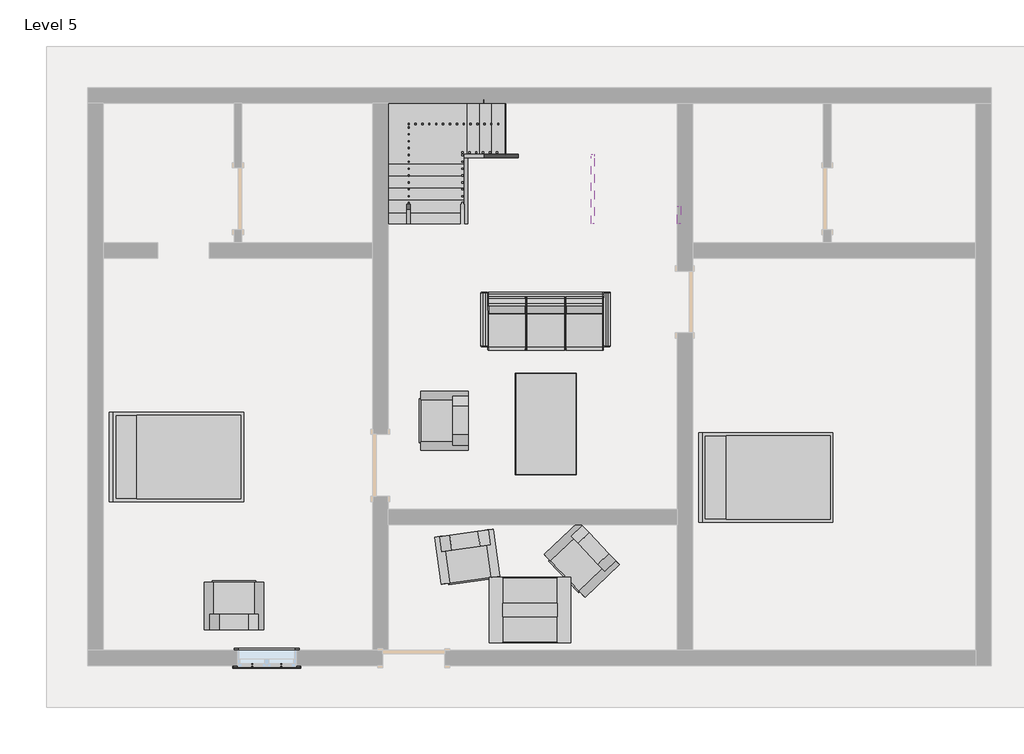
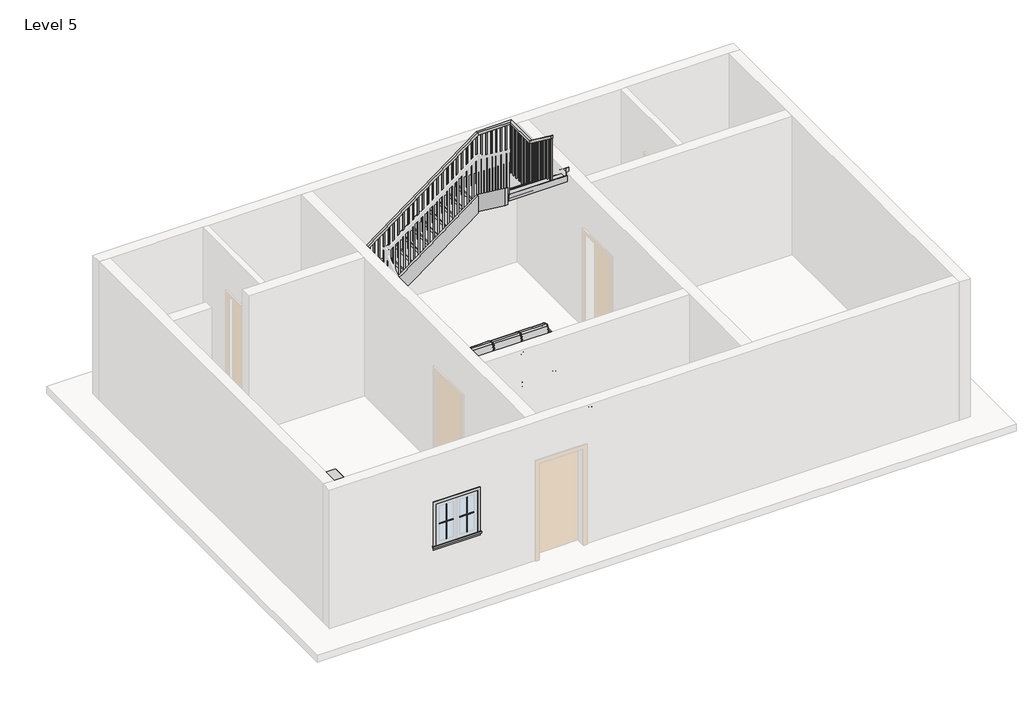
# One storey, part 2 of 2: 9 furniture elements, 6 members, 4 proxies, 1 railing, 1 stair flight.
"""IFC4 building model written with IfcOpenShell, lengths in millimetres."""

from ifc_helpers import new_model, si_unit, frame, origin, place, context, project, spatial, polyline, outline, extrude, faceted_brep, transform, mapped, element, save
from components import muntin_pattern_2x2_muntin_pattern_2x2_b3fe6957, muntin_pattern_2x2_muntin_pattern_2x2_3e0ecaf2, trim_window_exterior_flat_with_sill_41619996, trim_window_interior_flat_picture_frame_51c85655, furniture_2fc85b74, furniture_29a9adb8, furniture_57072a26, bed_17739_bed_17739_15c61121, chair_lounge_11461_couch_0866092f, dining_table_14755_dining_table_14755_d89cb775, wood_and_glass_coffee_table_17065_wood_and_glass_coffee_dbc724b2, stair_flight_e836c5a9

model = new_model("IFC4")

# Units and contexts
model_context = context("Model", 3, world=origin())
ifc_project = project(units=[si_unit("LENGTHUNIT", "METRE", prefix="MILLI")], contexts=[model_context])

# Site, building, storey
site = spatial("IfcSite", under=ifc_project)
building = spatial("IfcBuilding", under=site)
storey = spatial("IfcBuildingStorey", under=building, Name="Level 5", Elevation=9601.2)

# Proxies
placement = place(None, origin())
muntin_pattern_2x2_muntin_pattern_2x2_shape = muntin_pattern_2x2_muntin_pattern_2x2_b3fe6957(model_context)
element("IfcBuildingElementProxy", 1, Name="Muntin Pattern_2x2 : Muntin Pattern_2x2", ObjectType="Muntin Pattern_2x2 : Muntin Pattern_2x2", at=placement, inside=storey, context=model_context, shape_type="MappedRepresentation", body=[
    mapped(muntin_pattern_2x2_muntin_pattern_2x2_shape, transform((-5069.3921642, -1799.3582394, 10738.1934313), x_axis=(-1.0, 0.0, 0.0), y_axis=(0.0, -1.0, 0.0), z_axis=(0.0, 0.0, 1.0))),
])
muntin_pattern_2x2_muntin_pattern_2x2_2_shape = muntin_pattern_2x2_muntin_pattern_2x2_3e0ecaf2(model_context)
element("IfcBuildingElementProxy", 2, Name="Muntin Pattern_2x2 : Muntin Pattern_2x2", ObjectType="Muntin Pattern_2x2 : Muntin Pattern_2x2", at=placement, inside=storey, context=model_context, shape_type="MappedRepresentation", body=[
    mapped(muntin_pattern_2x2_muntin_pattern_2x2_2_shape, transform((-5498.0171642, -1799.3582394, 10738.1934313), x_axis=(1.0, 0.0, 0.0), y_axis=(0.0, 1.0, 0.0), z_axis=(0.0, 0.0, 1.0))),
])
trim_window_exterior_flat_with_sill_shape = trim_window_exterior_flat_with_sill_41619996(model_context)
element("IfcBuildingElementProxy", 3, Name="Trim-Window-Exterior-Flat : with Sill", ObjectType="Trim-Window-Exterior-Flat : with Sill", at=placement, inside=storey, context=model_context, shape_type="MappedRepresentation", body=[
    mapped(trim_window_exterior_flat_with_sill_shape, transform((-5283.7046642, -1808.8832394, 11582.7434313), x_axis=(1.0, 0.0, 0.0), y_axis=(0.0, 0.0, 1.0), z_axis=(0.0, -1.0, 0.0))),
])
trim_window_interior_flat_picture_frame_shape = trim_window_interior_flat_picture_frame_51c85655(model_context)
element("IfcBuildingElementProxy", 4, Name="Trim-Window-Interior-Flat : Picture Frame", ObjectType="Trim-Window-Interior-Flat : Picture Frame", at=placement, inside=storey, context=model_context, shape_type="MappedRepresentation", body=[
    mapped(trim_window_interior_flat_picture_frame_shape, transform((-5283.7046642, -1580.2832394, 11582.7434313), x_axis=(-1.0, 0.0, 0.0), y_axis=(0.0, 0.0, 1.0), z_axis=(0.0, 1.0, 0.0))),
])

# Furniture
furniture_shape = furniture_2fc85b74(model_context)
furniture_2_shape = furniture_29a9adb8(model_context)
furniture_3_shape = furniture_57072a26(model_context)
element("IfcFurniture", 5, at=placement, inside=storey, context=model_context, shape_type="MappedRepresentation", body=[
    mapped(furniture_shape, transform((-1166.392994, 2905.4688314, 9601.2), x_axis=(1.0, 0.0, 0.0), y_axis=(0.0, 1.0, 0.0), z_axis=(0.0, 0.0, 1.0))),
    mapped(furniture_2_shape, transform((-1166.392994, 2905.4688314, 9601.2), x_axis=(1.0, 0.0, 0.0), y_axis=(0.0, 1.0, 0.0), z_axis=(0.0, 0.0, 1.0))),
    mapped(furniture_3_shape, transform((-1166.392994, 2905.4688314, 9601.2), x_axis=(1.0, 0.0, 0.0), y_axis=(0.0, 1.0, 0.0), z_axis=(0.0, 0.0, 1.0))),
])
bed_17739_bed_17739_shape = bed_17739_bed_17739_15c61121(model_context)
element("IfcFurniture", 6, ObjectType="Bed_17739 : Bed_17739", at=placement, inside=storey, context=model_context, shape_type="MappedRepresentation", body=[
    mapped(bed_17739_bed_17739_shape, transform((-6591.8046642, 1277.2167606, 9601.2), x_axis=(0.0, 1.0, 0.0), y_axis=(-1.0, 0.0, 0.0), z_axis=(0.0, 0.0, 1.0))),
])
element("IfcFurniture", 7, ObjectType="Bed_17739 : Bed_17739", at=placement, inside=storey, context=model_context, shape_type="MappedRepresentation", body=[
    mapped(bed_17739_bed_17739_shape, transform((2107.6953358, 972.4167606, 9601.2), x_axis=(0.0, 1.0, 0.0), y_axis=(-1.0, 0.0, 0.0), z_axis=(0.0, 0.0, 1.0))),
])
chair_lounge_11461_couch_shape = chair_lounge_11461_couch_0866092f(model_context)
element("IfcFurniture", 8, ObjectType="Chair-Lounge_11461 : Couch", at=placement, inside=storey, context=model_context, shape_type="MappedRepresentation", body=[
    mapped(chair_lounge_11461_couch_shape, transform((-5766.3046642, -1273.9095448, 9601.2), x_axis=(-1.0, 0.0, 0.0), y_axis=(0.0, -1.0, 0.0), z_axis=(0.0, 0.0, 1.0))),
])
element("IfcFurniture", 9, ObjectType="Chair-Lounge_11461 : Couch", at=placement, inside=storey, context=model_context, shape_type="MappedRepresentation", body=[
    mapped(chair_lounge_11461_couch_shape, transform((-2311.9046642, 1810.6167606, 9601.2), x_axis=(0.0, -1.0, 0.0), y_axis=(1.0, 0.0, 0.0), z_axis=(0.0, 0.0, 1.0))),
])
element("IfcFurniture", 10, ObjectType="Chair-Lounge_11461 : Couch", at=placement, inside=storey, context=model_context, shape_type="MappedRepresentation", body=[
    mapped(chair_lounge_11461_couch_shape, transform((-2372.9488995, 149.9169276, 9601.2), x_axis=(0.9905324493396854, 0.1372787922627668, 0.0), y_axis=(-0.1372787922627668, 0.9905324493396854, 0.0), z_axis=(0.0, 0.0, 1.0))),
])
element("IfcFurniture", 11, ObjectType="Chair-Lounge_11461 : Couch", at=placement, inside=storey, context=model_context, shape_type="MappedRepresentation", body=[
    mapped(chair_lounge_11461_couch_shape, transform((-378.7925234, 1.7617886, 9601.2), x_axis=(0.6894995564131732, -0.7242861048688133, 0.0), y_axis=(0.7242861048688133, 0.6894995564131732, 0.0), z_axis=(0.0, 0.0, 1.0))),
])
dining_table_14755_dining_table_14755_shape = dining_table_14755_dining_table_14755_d89cb775(model_context)
element("IfcFurniture", 12, ObjectType="Dining_table_14755 : Dining_table_14755", at=placement, inside=storey, context=model_context, shape_type="MappedRepresentation", body=[
    mapped(dining_table_14755_dining_table_14755_shape, transform((-711.7046642, 1010.5167606, 9601.2), x_axis=(0.0, 1.0, 0.0), y_axis=(-1.0, 0.0, 0.0), z_axis=(0.0, 0.0, 1.0))),
])
wood_and_glass_coffee_table_17065_wood_and_glass_coffee_shape = wood_and_glass_coffee_table_17065_wood_and_glass_coffee_dbc724b2(model_context)
element("IfcFurniture", 13, ObjectType="Wood_and_Glass_Coffee_Table_17065 : Wood_and_Glass_Coffee_Table_17065", at=placement, inside=storey, context=model_context, shape_type="MappedRepresentation", body=[
    mapped(wood_and_glass_coffee_table_17065_wood_and_glass_coffee_shape, transform((-1397.5046642, -983.3832394, 9601.2), x_axis=(1.0, 0.0, 0.0), y_axis=(0.0, 1.0, 0.0), z_axis=(0.0, 0.0, 1.0))),
])

# Members
element("IfcMember", 14, ObjectType="Stringer - 2\" Width", at=placement, inside=storey, context=model_context, shape_type="SweptSolid", body=[
    extrude(outline(polyline([(4718.9167606, 9601.2), (4718.9167606, 9748.8508226), (5113.281957, 9748.8508226), (4911.6463024, 9601.2), (4718.9167606, 9601.2)])), frame((-3543.8046642, 0.0, 0.0), z_axis=(1.0, 0.0, 0.0), x_axis=(0.0, 1.0, 0.0)), (0.0, 0.0, 1.0), 50.8),
])
element("IfcMember", 15, ObjectType="Stringer - 2\" Width", at=placement, inside=storey, context=model_context, shape_type="SweptSolid", body=[
    extrude(outline(polyline([(10762.0387795, -1623.6098785), (11417.9484291, -743.5977653), (11417.9484291, -1253.6320422), (10762.0387795, -2133.6441554), (10762.0387795, -1623.6098785)])), frame((0.0, 6496.9167606, 0.0), z_axis=(0.0, 1.0, 0.0), x_axis=(0.0, 0.0, 1.0)), (0.0, 0.0, 1.0), 50.8),
])
element("IfcMember", 16, ObjectType="Stringer - 2\" Width", at=placement, inside=storey, context=model_context, shape_type="SweptSolid", body=[
    extrude(outline(polyline([(4718.9167606, 12549.2227901), (4718.9167606, 12743.1652405), (4979.1229954, 12549.2227901), (4718.9167606, 12549.2227901)])), frame((774.1953358, 0.0, 0.0), z_axis=(1.0, 0.0, 0.0), x_axis=(0.0, 1.0, 0.0)), (0.0, 0.0, 1.0), 50.8),
])
element("IfcMember", 17, ObjectType="Stringer - 2\" Width", at=placement, inside=storey, context=model_context, shape_type="SweptSolid", body=[
    extrude(outline(polyline([(4718.9167606, 9601.2), (4718.9167606, 9837.8522719), (5695.7536537, 10553.1561753), (5695.7536537, 10175.3747195), (4911.6463024, 9601.2), (4718.9167606, 9601.2)])), frame((-2368.6972892, 0.0, 0.0), z_axis=(1.0, 0.0, 0.0), x_axis=(0.0, 1.0, 0.0)), (0.0, 0.0, 1.0), 50.8),
])
element("IfcMember", 18, ObjectType="Stringer - 2\" Width", at=placement, inside=storey, context=model_context, shape_type="SweptSolid", body=[
    extrude(outline(polyline([(10586.8438971, -2368.6972892), (10212.5738041, -2368.6972892), (10212.5738041, -2360.8087204), (11602.6389392, -495.8046642), (11977.2250342, -495.8046642), (11977.2250342, -503.2692636), (10586.8438971, -2368.6972892)])), frame((0.0, 5695.7536537, 0.0), z_axis=(0.0, 1.0, 0.0), x_axis=(0.0, 0.0, 1.0)), (0.0, 0.0, 1.0), 50.8),
])
element("IfcMember", 19, ObjectType="Stringer - 2\" Width", at=placement, inside=storey, context=model_context, shape_type="SweptSolid", body=[
    extrude(outline(polyline([(5746.5536537, 11977.2250342), (5746.5536537, 11640.5022932), (5688.2891085, 11640.5022932), (4718.9167606, 12363.0155283), (4718.9167606, 12743.1652405), (5746.5536537, 11977.2250342)])), frame((-495.8046642, 0.0, 0.0), z_axis=(1.0, 0.0, 0.0), x_axis=(0.0, 1.0, 0.0)), (0.0, 0.0, 1.0), 50.8),
])

# Railing
element("IfcRailing", 20, ObjectType="Handrail - Rectangular", at=placement, inside=storey, context=model_context, shape_type="SolidModel", body=[
    faceted_brep([(-3213.6046642, 4718.9167606, 10648.1217391), (-3213.6046642, 4718.9167606, 10584.7634439), (-3162.8046642, 4718.9167606, 10584.7634439), (-3162.8046642, 4718.9167606, 10648.1217391), (-3213.6046642, 5555.0306195, 11271.312193), (-3213.6046642, 5571.8796657, 11220.512193), (-3162.8046642, 5571.8796657, 11220.512193), (-3162.8046642, 5555.0306195, 11271.312193), (-3213.6046642, 6217.5167606, 11271.312193), (-3213.6046642, 6217.5167606, 11220.512193), (-3162.8046642, 6166.7167606, 11220.512193), (-3162.8046642, 6166.7167606, 11271.312193), (-2551.1185231, 6217.5167606, 11271.312193), (-2534.269477, 6217.5167606, 11220.512193), (-2534.269477, 6166.7167606, 11220.512193), (-2551.1185231, 6166.7167606, 11271.312193), (-239.7185231, 6217.5167606, 12994.0948017), (-222.869477, 6217.5167606, 12943.2948017), (-222.869477, 6166.7167606, 12943.2948017), (-239.7185231, 6166.7167606, 12994.0948017), (494.7953358, 6217.5167606, 12994.0948017), (494.7953358, 6217.5167606, 12943.2948017), (443.9953358, 6166.7167606, 12943.2948017), (443.9953358, 6166.7167606, 12994.0948017), (494.7953358, 5483.0029017, 12994.0948017), (494.7953358, 5466.1538556, 12943.2948017), (443.9953358, 5466.1538556, 12943.2948017), (443.9953358, 5483.0029017, 12994.0948017), (494.7953358, 4718.9167606, 13563.6), (443.9953358, 4718.9167606, 13563.6), (443.9953358, 4718.9167606, 13500.2417047), (494.7953358, 4718.9167606, 13500.2417047)], [[[0, 1, 2, 3]], [[1, 0, 4, 5]], [[2, 1, 5, 6]], [[3, 2, 6, 7]], [[0, 3, 7, 4]], [[5, 4, 8, 9]], [[6, 5, 9, 10]], [[7, 6, 10, 11]], [[4, 7, 11, 8]], [[9, 8, 12, 13]], [[10, 9, 13, 14]], [[11, 10, 14, 15]], [[8, 11, 15, 12]], [[13, 12, 16, 17]], [[14, 13, 17, 18]], [[15, 14, 18, 19]], [[12, 15, 19, 16]], [[17, 16, 20, 21]], [[18, 17, 21, 22]], [[19, 18, 22, 23]], [[16, 19, 23, 20]], [[21, 20, 24, 25]], [[22, 21, 25, 26]], [[23, 22, 26, 27]], [[20, 23, 27, 24]], [[28, 29, 30, 31]], [[25, 24, 28, 31]], [[26, 25, 31, 30]], [[27, 26, 30, 29]], [[24, 27, 29, 28]]]),
    extrude(outline(polyline([(4779.2417606, 13455.2789718), (4779.2417606, 12516.6782609), (4760.1917606, 12516.6782609), (4760.1917606, 13469.4777296), (4779.2417606, 13455.2789718)])), frame((459.8703358, 0.0, 0.0), z_axis=(1.0, 0.0, 0.0), x_axis=(0.0, 1.0, 0.0)), (0.0, 0.0, 1.0), 19.05),
    extrude(outline(polyline([(4880.8417606, 13379.5522637), (4880.8417606, 12516.6782609), (4861.7917606, 12516.6782609), (4861.7917606, 13393.7510215), (4880.8417606, 13379.5522637)])), frame((459.8703358, 0.0, 0.0), z_axis=(1.0, 0.0, 0.0), x_axis=(0.0, 1.0, 0.0)), (0.0, 0.0, 1.0), 19.05),
    extrude(outline(polyline([(4982.4417606, 13303.8255557), (4982.4417606, 12384.1565217), (4963.3917606, 12384.1565217), (4963.3917606, 13318.0243134), (4982.4417606, 13303.8255557)])), frame((459.8703358, 0.0, 0.0), z_axis=(1.0, 0.0, 0.0), x_axis=(0.0, 1.0, 0.0)), (0.0, 0.0, 1.0), 19.05),
    extrude(outline(polyline([(5084.0417606, 13228.0988476), (5084.0417606, 12384.1565217), (5064.9917606, 12384.1565217), (5064.9917606, 13242.2976054), (5084.0417606, 13228.0988476)])), frame((459.8703358, 0.0, 0.0), z_axis=(1.0, 0.0, 0.0), x_axis=(0.0, 1.0, 0.0)), (0.0, 0.0, 1.0), 19.05),
    extrude(outline(polyline([(5185.6417606, 13152.3721395), (5185.6417606, 12251.6347826), (5166.5917606, 12251.6347826), (5166.5917606, 13166.5708973), (5185.6417606, 13152.3721395)])), frame((459.8703358, 0.0, 0.0), z_axis=(1.0, 0.0, 0.0), x_axis=(0.0, 1.0, 0.0)), (0.0, 0.0, 1.0), 19.05),
    extrude(outline(polyline([(5287.2417606, 13076.6454314), (5287.2417606, 12119.1130435), (5268.1917606, 12119.1130435), (5268.1917606, 13090.8441892), (5287.2417606, 13076.6454314)])), frame((459.8703358, 0.0, 0.0), z_axis=(1.0, 0.0, 0.0), x_axis=(0.0, 1.0, 0.0)), (0.0, 0.0, 1.0), 19.05),
    extrude(outline(polyline([(5388.8417606, 13000.9187234), (5388.8417606, 12119.1130435), (5369.7917606, 12119.1130435), (5369.7917606, 13015.1174811), (5388.8417606, 13000.9187234)])), frame((459.8703358, 0.0, 0.0), z_axis=(1.0, 0.0, 0.0), x_axis=(0.0, 1.0, 0.0)), (0.0, 0.0, 1.0), 19.05),
    extrude(outline(polyline([(5490.4417606, 12925.1920153), (5490.4417606, 11986.5913043), (5471.3917606, 11986.5913043), (5471.3917606, 12939.3907731), (5490.4417606, 12925.1920153)])), frame((459.8703358, 0.0, 0.0), z_axis=(1.0, 0.0, 0.0), x_axis=(0.0, 1.0, 0.0)), (0.0, 0.0, 1.0), 19.05),
    extrude(outline(polyline([(478.9203358, 5592.0417606), (478.9203358, 5572.9917606), (459.8703358, 5572.9917606), (459.8703358, 5592.0417606), (478.9203358, 5592.0417606)])), frame((0.0, 0.0, 11986.5913043), z_axis=(0.0, 0.0, 1.0), x_axis=(1.0, 0.0, 0.0)), (0.0, 0.0, 1.0), 956.7034973),
    extrude(outline(polyline([(478.9203358, 5693.6417606), (478.9203358, 5674.5917606), (459.8703358, 5674.5917606), (459.8703358, 5693.6417606), (478.9203358, 5693.6417606)])), frame((0.0, 0.0, 11854.0695652), z_axis=(0.0, 0.0, 1.0), x_axis=(1.0, 0.0, 0.0)), (0.0, 0.0, 1.0), 1089.2252364),
    extrude(outline(polyline([(478.9203358, 5795.2417606), (478.9203358, 5776.1917606), (459.8703358, 5776.1917606), (459.8703358, 5795.2417606), (478.9203358, 5795.2417606)])), frame((0.0, 0.0, 11854.0695652), z_axis=(0.0, 0.0, 1.0), x_axis=(1.0, 0.0, 0.0)), (0.0, 0.0, 1.0), 1089.2252364),
    extrude(outline(polyline([(478.9203358, 5896.8417606), (478.9203358, 5877.7917606), (459.8703358, 5877.7917606), (459.8703358, 5896.8417606), (478.9203358, 5896.8417606)])), frame((0.0, 0.0, 11854.0695652), z_axis=(0.0, 0.0, 1.0), x_axis=(1.0, 0.0, 0.0)), (0.0, 0.0, 1.0), 1089.2252364),
    extrude(outline(polyline([(478.9203358, 5998.4417606), (478.9203358, 5979.3917606), (459.8703358, 5979.3917606), (459.8703358, 5998.4417606), (478.9203358, 5998.4417606)])), frame((0.0, 0.0, 11854.0695652), z_axis=(0.0, 0.0, 1.0), x_axis=(1.0, 0.0, 0.0)), (0.0, 0.0, 1.0), 1089.2252364),
    extrude(outline(polyline([(478.9203358, 6100.0417606), (478.9203358, 6080.9917606), (459.8703358, 6080.9917606), (459.8703358, 6100.0417606), (478.9203358, 6100.0417606)])), frame((0.0, 0.0, 11854.0695652), z_axis=(0.0, 0.0, 1.0), x_axis=(1.0, 0.0, 0.0)), (0.0, 0.0, 1.0), 1089.2252364),
    extrude(outline(polyline([(358.2703358, 6201.6417606), (377.3203358, 6201.6417606), (377.3203358, 6182.5917606), (358.2703358, 6182.5917606), (358.2703358, 6201.6417606)])), frame((0.0, 0.0, 11854.0695652), z_axis=(0.0, 0.0, 1.0), x_axis=(1.0, 0.0, 0.0)), (0.0, 0.0, 1.0), 1089.2252364),
    extrude(outline(polyline([(256.6703358, 6201.6417606), (275.7203358, 6201.6417606), (275.7203358, 6182.5917606), (256.6703358, 6182.5917606), (256.6703358, 6201.6417606)])), frame((0.0, 0.0, 11854.0695652), z_axis=(0.0, 0.0, 1.0), x_axis=(1.0, 0.0, 0.0)), (0.0, 0.0, 1.0), 1089.2252364),
    extrude(outline(polyline([(155.0703358, 6201.6417606), (174.1203358, 6201.6417606), (174.1203358, 6182.5917606), (155.0703358, 6182.5917606), (155.0703358, 6201.6417606)])), frame((0.0, 0.0, 11854.0695652), z_axis=(0.0, 0.0, 1.0), x_axis=(1.0, 0.0, 0.0)), (0.0, 0.0, 1.0), 1089.2252364),
    extrude(outline(polyline([(53.4703358, 6201.6417606), (72.5203358, 6201.6417606), (72.5203358, 6182.5917606), (53.4703358, 6182.5917606), (53.4703358, 6201.6417606)])), frame((0.0, 0.0, 11854.0695652), z_axis=(0.0, 0.0, 1.0), x_axis=(1.0, 0.0, 0.0)), (0.0, 0.0, 1.0), 1089.2252364),
    extrude(outline(polyline([(-48.1296642, 6201.6417606), (-29.0796642, 6201.6417606), (-29.0796642, 6182.5917606), (-48.1296642, 6182.5917606), (-48.1296642, 6201.6417606)])), frame((0.0, 0.0, 11854.0695652), z_axis=(0.0, 0.0, 1.0), x_axis=(1.0, 0.0, 0.0)), (0.0, 0.0, 1.0), 1089.2252364),
    extrude(outline(polyline([(-149.7296642, 6201.6417606), (-130.6796642, 6201.6417606), (-130.6796642, 6182.5917606), (-149.7296642, 6182.5917606), (-149.7296642, 6201.6417606)])), frame((0.0, 0.0, 11854.0695652), z_axis=(0.0, 0.0, 1.0), x_axis=(1.0, 0.0, 0.0)), (0.0, 0.0, 1.0), 1089.2252364),
    extrude(outline(polyline([(12922.0822397, -251.3296642), (11854.0695652, -251.3296642), (11854.0695652, -232.2796642), (12936.2809975, -232.2796642), (12922.0822397, -251.3296642)])), frame((0.0, 6182.5917606, 0.0), z_axis=(0.0, 1.0, 0.0), x_axis=(0.0, 0.0, 1.0)), (0.0, 0.0, 1.0), 19.05),
    extrude(outline(polyline([(12846.3555316, -352.9296642), (11854.0695652, -352.9296642), (11854.0695652, -333.8796642), (12860.5542894, -333.8796642), (12846.3555316, -352.9296642)])), frame((0.0, 6182.5917606, 0.0), z_axis=(0.0, 1.0, 0.0), x_axis=(0.0, 0.0, 1.0)), (0.0, 0.0, 1.0), 19.05),
    extrude(outline(polyline([(12770.6288236, -454.5296642), (11854.0695652, -454.5296642), (11854.0695652, -435.4796642), (12784.8275813, -435.4796642), (12770.6288236, -454.5296642)])), frame((0.0, 6182.5917606, 0.0), z_axis=(0.0, 1.0, 0.0), x_axis=(0.0, 0.0, 1.0)), (0.0, 0.0, 1.0), 19.05),
    extrude(outline(polyline([(12694.9021155, -556.1296642), (11721.5478261, -556.1296642), (11721.5478261, -537.0796642), (12709.1008733, -537.0796642), (12694.9021155, -556.1296642)])), frame((0.0, 6182.5917606, 0.0), z_axis=(0.0, 1.0, 0.0), x_axis=(0.0, 0.0, 1.0)), (0.0, 0.0, 1.0), 19.05),
    extrude(outline(polyline([(12619.1754074, -657.7296642), (11721.5478261, -657.7296642), (11721.5478261, -638.6796642), (12633.3741652, -638.6796642), (12619.1754074, -657.7296642)])), frame((0.0, 6182.5917606, 0.0), z_axis=(0.0, 1.0, 0.0), x_axis=(0.0, 0.0, 1.0)), (0.0, 0.0, 1.0), 19.05),
    extrude(outline(polyline([(12543.4486993, -759.3296642), (11589.026087, -759.3296642), (11589.026087, -740.2796642), (12557.6474571, -740.2796642), (12543.4486993, -759.3296642)])), frame((0.0, 6182.5917606, 0.0), z_axis=(0.0, 1.0, 0.0), x_axis=(0.0, 0.0, 1.0)), (0.0, 0.0, 1.0), 19.05),
    extrude(outline(polyline([(12467.7219913, -860.9296642), (11589.026087, -860.9296642), (11589.026087, -841.8796642), (12481.920749, -841.8796642), (12467.7219913, -860.9296642)])), frame((0.0, 6182.5917606, 0.0), z_axis=(0.0, 1.0, 0.0), x_axis=(0.0, 0.0, 1.0)), (0.0, 0.0, 1.0), 19.05),
    extrude(outline(polyline([(12391.9952832, -962.5296642), (11456.5043478, -962.5296642), (11456.5043478, -943.4796642), (12406.194041, -943.4796642), (12391.9952832, -962.5296642)])), frame((0.0, 6182.5917606, 0.0), z_axis=(0.0, 1.0, 0.0), x_axis=(0.0, 0.0, 1.0)), (0.0, 0.0, 1.0), 19.05),
    extrude(outline(polyline([(12316.2685751, -1064.1296642), (11456.5043478, -1064.1296642), (11456.5043478, -1045.0796642), (12330.4673329, -1045.0796642), (12316.2685751, -1064.1296642)])), frame((0.0, 6182.5917606, 0.0), z_axis=(0.0, 1.0, 0.0), x_axis=(0.0, 0.0, 1.0)), (0.0, 0.0, 1.0), 19.05),
    extrude(outline(polyline([(12240.541867, -1165.7296642), (11323.9826087, -1165.7296642), (11323.9826087, -1146.6796642), (12254.7406248, -1146.6796642), (12240.541867, -1165.7296642)])), frame((0.0, 6182.5917606, 0.0), z_axis=(0.0, 1.0, 0.0), x_axis=(0.0, 0.0, 1.0)), (0.0, 0.0, 1.0), 19.05),
    extrude(outline(polyline([(12164.815159, -1267.3296642), (11191.4608696, -1267.3296642), (11191.4608696, -1248.2796642), (12179.0139167, -1248.2796642), (12164.815159, -1267.3296642)])), frame((0.0, 6182.5917606, 0.0), z_axis=(0.0, 1.0, 0.0), x_axis=(0.0, 0.0, 1.0)), (0.0, 0.0, 1.0), 19.05),
    extrude(outline(polyline([(12089.0884509, -1368.9296642), (11191.4608696, -1368.9296642), (11191.4608696, -1349.8796642), (12103.2872087, -1349.8796642), (12089.0884509, -1368.9296642)])), frame((0.0, 6182.5917606, 0.0), z_axis=(0.0, 1.0, 0.0), x_axis=(0.0, 0.0, 1.0)), (0.0, 0.0, 1.0), 19.05),
    extrude(outline(polyline([(12013.3617428, -1470.5296642), (11058.9391304, -1470.5296642), (11058.9391304, -1451.4796642), (12027.5605006, -1451.4796642), (12013.3617428, -1470.5296642)])), frame((0.0, 6182.5917606, 0.0), z_axis=(0.0, 1.0, 0.0), x_axis=(0.0, 0.0, 1.0)), (0.0, 0.0, 1.0), 19.05),
    extrude(outline(polyline([(11937.6350347, -1572.1296642), (11058.9391304, -1572.1296642), (11058.9391304, -1553.0796642), (11951.8337925, -1553.0796642), (11937.6350347, -1572.1296642)])), frame((0.0, 6182.5917606, 0.0), z_axis=(0.0, 1.0, 0.0), x_axis=(0.0, 0.0, 1.0)), (0.0, 0.0, 1.0), 19.05),
    extrude(outline(polyline([(11861.9083267, -1673.7296642), (10926.4173913, -1673.7296642), (10926.4173913, -1654.6796642), (11876.1070844, -1654.6796642), (11861.9083267, -1673.7296642)])), frame((0.0, 6182.5917606, 0.0), z_axis=(0.0, 1.0, 0.0), x_axis=(0.0, 0.0, 1.0)), (0.0, 0.0, 1.0), 19.05),
    extrude(outline(polyline([(11786.1816186, -1775.3296642), (10926.4173913, -1775.3296642), (10926.4173913, -1756.2796642), (11800.3803764, -1756.2796642), (11786.1816186, -1775.3296642)])), frame((0.0, 6182.5917606, 0.0), z_axis=(0.0, 1.0, 0.0), x_axis=(0.0, 0.0, 1.0)), (0.0, 0.0, 1.0), 19.05),
    extrude(outline(polyline([(11710.4549105, -1876.9296642), (10793.8956522, -1876.9296642), (10793.8956522, -1857.8796642), (11724.6536683, -1857.8796642), (11710.4549105, -1876.9296642)])), frame((0.0, 6182.5917606, 0.0), z_axis=(0.0, 1.0, 0.0), x_axis=(0.0, 0.0, 1.0)), (0.0, 0.0, 1.0), 19.05),
    extrude(outline(polyline([(11634.7282025, -1978.5296642), (10661.373913, -1978.5296642), (10661.373913, -1959.4796642), (11648.9269602, -1959.4796642), (11634.7282025, -1978.5296642)])), frame((0.0, 6182.5917606, 0.0), z_axis=(0.0, 1.0, 0.0), x_axis=(0.0, 0.0, 1.0)), (0.0, 0.0, 1.0), 19.05),
    extrude(outline(polyline([(11559.0014944, -2080.1296642), (10661.373913, -2080.1296642), (10661.373913, -2061.0796642), (11573.2002521, -2061.0796642), (11559.0014944, -2080.1296642)])), frame((0.0, 6182.5917606, 0.0), z_axis=(0.0, 1.0, 0.0), x_axis=(0.0, 0.0, 1.0)), (0.0, 0.0, 1.0), 19.05),
    extrude(outline(polyline([(11483.2747863, -2181.7296642), (10528.8521739, -2181.7296642), (10528.8521739, -2162.6796642), (11497.4735441, -2162.6796642), (11483.2747863, -2181.7296642)])), frame((0.0, 6182.5917606, 0.0), z_axis=(0.0, 1.0, 0.0), x_axis=(0.0, 0.0, 1.0)), (0.0, 0.0, 1.0), 19.05),
    extrude(outline(polyline([(11407.5480782, -2283.3296642), (10528.8521739, -2283.3296642), (10528.8521739, -2264.2796642), (11421.746836, -2264.2796642), (11407.5480782, -2283.3296642)])), frame((0.0, 6182.5917606, 0.0), z_axis=(0.0, 1.0, 0.0), x_axis=(0.0, 0.0, 1.0)), (0.0, 0.0, 1.0), 19.05),
    extrude(outline(polyline([(11331.8213702, -2384.9296642), (10396.3304348, -2384.9296642), (10396.3304348, -2365.8796642), (11346.0201279, -2365.8796642), (11331.8213702, -2384.9296642)])), frame((0.0, 6182.5917606, 0.0), z_axis=(0.0, 1.0, 0.0), x_axis=(0.0, 0.0, 1.0)), (0.0, 0.0, 1.0), 19.05),
    extrude(outline(polyline([(11256.0946621, -2486.5296642), (10396.3304348, -2486.5296642), (10396.3304348, -2467.4796642), (11270.2934198, -2467.4796642), (11256.0946621, -2486.5296642)])), frame((0.0, 6182.5917606, 0.0), z_axis=(0.0, 1.0, 0.0), x_axis=(0.0, 0.0, 1.0)), (0.0, 0.0, 1.0), 19.05),
    extrude(outline(polyline([(-2588.1296642, 6201.6417606), (-2569.0796642, 6201.6417606), (-2569.0796642, 6182.5917606), (-2588.1296642, 6182.5917606), (-2588.1296642, 6201.6417606)])), frame((0.0, 0.0, 10396.3304348), z_axis=(0.0, 0.0, 1.0), x_axis=(1.0, 0.0, 0.0)), (0.0, 0.0, 1.0), 824.1817582),
    extrude(outline(polyline([(-2689.7296642, 6201.6417606), (-2670.6796642, 6201.6417606), (-2670.6796642, 6182.5917606), (-2689.7296642, 6182.5917606), (-2689.7296642, 6201.6417606)])), frame((0.0, 0.0, 10396.3304348), z_axis=(0.0, 0.0, 1.0), x_axis=(1.0, 0.0, 0.0)), (0.0, 0.0, 1.0), 824.1817582),
    extrude(outline(polyline([(-2791.3296642, 6201.6417606), (-2772.2796642, 6201.6417606), (-2772.2796642, 6182.5917606), (-2791.3296642, 6182.5917606), (-2791.3296642, 6201.6417606)])), frame((0.0, 0.0, 10396.3304348), z_axis=(0.0, 0.0, 1.0), x_axis=(1.0, 0.0, 0.0)), (0.0, 0.0, 1.0), 824.1817582),
    extrude(outline(polyline([(-2892.9296642, 6201.6417606), (-2873.8796642, 6201.6417606), (-2873.8796642, 6182.5917606), (-2892.9296642, 6182.5917606), (-2892.9296642, 6201.6417606)])), frame((0.0, 0.0, 10396.3304348), z_axis=(0.0, 0.0, 1.0), x_axis=(1.0, 0.0, 0.0)), (0.0, 0.0, 1.0), 824.1817582),
    extrude(outline(polyline([(-2994.5296642, 6201.6417606), (-2975.4796642, 6201.6417606), (-2975.4796642, 6182.5917606), (-2994.5296642, 6182.5917606), (-2994.5296642, 6201.6417606)])), frame((0.0, 0.0, 10396.3304348), z_axis=(0.0, 0.0, 1.0), x_axis=(1.0, 0.0, 0.0)), (0.0, 0.0, 1.0), 824.1817582),
    extrude(outline(polyline([(-3096.1296642, 6201.6417606), (-3077.0796642, 6201.6417606), (-3077.0796642, 6182.5917606), (-3096.1296642, 6182.5917606), (-3096.1296642, 6201.6417606)])), frame((0.0, 0.0, 10396.3304348), z_axis=(0.0, 0.0, 1.0), x_axis=(1.0, 0.0, 0.0)), (0.0, 0.0, 1.0), 824.1817582),
    extrude(outline(polyline([(-3197.7296642, 6131.7917606), (-3197.7296642, 6150.8417606), (-3178.6796642, 6150.8417606), (-3178.6796642, 6131.7917606), (-3197.7296642, 6131.7917606)])), frame((0.0, 0.0, 10396.3304348), z_axis=(0.0, 0.0, 1.0), x_axis=(1.0, 0.0, 0.0)), (0.0, 0.0, 1.0), 824.1817582),
    extrude(outline(polyline([(-3197.7296642, 6030.1917606), (-3197.7296642, 6049.2417606), (-3178.6796642, 6049.2417606), (-3178.6796642, 6030.1917606), (-3197.7296642, 6030.1917606)])), frame((0.0, 0.0, 10396.3304348), z_axis=(0.0, 0.0, 1.0), x_axis=(1.0, 0.0, 0.0)), (0.0, 0.0, 1.0), 824.1817582),
    extrude(outline(polyline([(-3197.7296642, 5928.5917606), (-3197.7296642, 5947.6417606), (-3178.6796642, 5947.6417606), (-3178.6796642, 5928.5917606), (-3197.7296642, 5928.5917606)])), frame((0.0, 0.0, 10396.3304348), z_axis=(0.0, 0.0, 1.0), x_axis=(1.0, 0.0, 0.0)), (0.0, 0.0, 1.0), 824.1817582),
    extrude(outline(polyline([(-3197.7296642, 5826.9917606), (-3197.7296642, 5846.0417606), (-3178.6796642, 5846.0417606), (-3178.6796642, 5826.9917606), (-3197.7296642, 5826.9917606)])), frame((0.0, 0.0, 10396.3304348), z_axis=(0.0, 0.0, 1.0), x_axis=(1.0, 0.0, 0.0)), (0.0, 0.0, 1.0), 824.1817582),
    extrude(outline(polyline([(-3197.7296642, 5725.3917606), (-3197.7296642, 5744.4417606), (-3178.6796642, 5744.4417606), (-3178.6796642, 5725.3917606), (-3197.7296642, 5725.3917606)])), frame((0.0, 0.0, 10396.3304348), z_axis=(0.0, 0.0, 1.0), x_axis=(1.0, 0.0, 0.0)), (0.0, 0.0, 1.0), 824.1817582),
    extrude(outline(polyline([(-3197.7296642, 5623.7917606), (-3197.7296642, 5642.8417606), (-3178.6796642, 5642.8417606), (-3178.6796642, 5623.7917606), (-3197.7296642, 5623.7917606)])), frame((0.0, 0.0, 10396.3304348), z_axis=(0.0, 0.0, 1.0), x_axis=(1.0, 0.0, 0.0)), (0.0, 0.0, 1.0), 824.1817582),
    extrude(outline(polyline([(5541.2417606, 11197.6764873), (5541.2417606, 10263.8086957), (5522.1917606, 10263.8086957), (5522.1917606, 11183.4777296), (5541.2417606, 11197.6764873)])), frame((-3197.7296642, 0.0, 0.0), z_axis=(1.0, 0.0, 0.0), x_axis=(0.0, 1.0, 0.0)), (0.0, 0.0, 1.0), 19.05),
    extrude(outline(polyline([(5439.6417606, 11121.9497793), (5439.6417606, 10263.8086957), (5420.5917606, 10263.8086957), (5420.5917606, 11107.7510215), (5439.6417606, 11121.9497793)])), frame((-3197.7296642, 0.0, 0.0), z_axis=(1.0, 0.0, 0.0), x_axis=(0.0, 1.0, 0.0)), (0.0, 0.0, 1.0), 19.05),
    extrude(outline(polyline([(5338.0417606, 11046.2230712), (5338.0417606, 10131.2869565), (5318.9917606, 10131.2869565), (5318.9917606, 11032.0243134), (5338.0417606, 11046.2230712)])), frame((-3197.7296642, 0.0, 0.0), z_axis=(1.0, 0.0, 0.0), x_axis=(0.0, 1.0, 0.0)), (0.0, 0.0, 1.0), 19.05),
    extrude(outline(polyline([(5236.4417606, 10970.4963631), (5236.4417606, 9998.7652174), (5217.3917606, 9998.7652174), (5217.3917606, 10956.2976054), (5236.4417606, 10970.4963631)])), frame((-3197.7296642, 0.0, 0.0), z_axis=(1.0, 0.0, 0.0), x_axis=(0.0, 1.0, 0.0)), (0.0, 0.0, 1.0), 19.05),
    extrude(outline(polyline([(5134.8417606, 10894.769655), (5134.8417606, 9998.7652174), (5115.7917606, 9998.7652174), (5115.7917606, 10880.5708973), (5134.8417606, 10894.769655)])), frame((-3197.7296642, 0.0, 0.0), z_axis=(1.0, 0.0, 0.0), x_axis=(0.0, 1.0, 0.0)), (0.0, 0.0, 1.0), 19.05),
    extrude(outline(polyline([(5033.2417606, 10819.042947), (5033.2417606, 9866.2434783), (5014.1917606, 9866.2434783), (5014.1917606, 10804.8441892), (5033.2417606, 10819.042947)])), frame((-3197.7296642, 0.0, 0.0), z_axis=(1.0, 0.0, 0.0), x_axis=(0.0, 1.0, 0.0)), (0.0, 0.0, 1.0), 19.05),
    extrude(outline(polyline([(4931.6417606, 10743.3162389), (4931.6417606, 9866.2434783), (4912.5917606, 9866.2434783), (4912.5917606, 10729.1174811), (4931.6417606, 10743.3162389)])), frame((-3197.7296642, 0.0, 0.0), z_axis=(1.0, 0.0, 0.0), x_axis=(0.0, 1.0, 0.0)), (0.0, 0.0, 1.0), 19.05),
    extrude(outline(polyline([(4830.0417606, 10667.5895308), (4830.0417606, 9733.7217391), (4810.9917606, 9733.7217391), (4810.9917606, 10653.3907731), (4830.0417606, 10667.5895308)])), frame((-3197.7296642, 0.0, 0.0), z_axis=(1.0, 0.0, 0.0), x_axis=(0.0, 1.0, 0.0)), (0.0, 0.0, 1.0), 19.05),
    extrude(outline(polyline([(459.8703358, 6201.6417606), (478.9203358, 6201.6417606), (478.9203358, 6182.5917606), (459.8703358, 6182.5917606), (459.8703358, 6201.6417606)])), frame((0.0, 0.0, 11854.0695652), z_axis=(0.0, 0.0, 1.0), x_axis=(1.0, 0.0, 0.0)), (0.0, 0.0, 1.0), 1089.2252364),
    extrude(outline(polyline([(-3197.7296642, 6182.5917606), (-3197.7296642, 6201.6417606), (-3178.6796642, 6201.6417606), (-3178.6796642, 6182.5917606), (-3197.7296642, 6182.5917606)])), frame((0.0, 0.0, 10396.3304348), z_axis=(0.0, 0.0, 1.0), x_axis=(1.0, 0.0, 0.0)), (0.0, 0.0, 1.0), 824.1817582),
    extrude(outline(polyline([(4737.9667606, 13486.042947), (4737.9667606, 12516.6782609), (4718.9167606, 12516.6782609), (4718.9167606, 13500.2417047), (4737.9667606, 13486.042947)])), frame((459.8703358, 0.0, 0.0), z_axis=(1.0, 0.0, 0.0), x_axis=(0.0, 1.0, 0.0)), (0.0, 0.0, 1.0), 19.05),
    extrude(outline(polyline([(4737.9667606, 10598.9622016), (4737.9667606, 9733.7217391), (4718.9167606, 9733.7217391), (4718.9167606, 10584.7634439), (4737.9667606, 10598.9622016)])), frame((-3197.7296642, 0.0, 0.0), z_axis=(1.0, 0.0, 0.0), x_axis=(0.0, 1.0, 0.0)), (0.0, 0.0, 1.0), 19.05),
])

# Stair flight
stair_flight_shape = stair_flight_e836c5a9(model_context)
element("IfcStairFlight", 21, ObjectType="2\" Tread 1\" Nosing 1/4\" Riser", at=placement, inside=storey, context=model_context, shape_type="MappedRepresentation", body=[
    mapped(stair_flight_shape, transform((0.0, 0.0, 0.0), x_axis=(1.0, 0.0, 0.0), y_axis=(0.0, 1.0, 0.0), z_axis=(0.0, 0.0, 1.0))),
])

save(model, "model.ifc")

# Revit data of these elements
# Type "Muntin Pattern_2x2 : Muntin Pattern_2x2"
#   Width [instance default] = 4' - 0"
#   Thickness = 0' - 0 1/2"
#   Height [instance default] = 4' - 0"
#   Distance = 0' - 0 3/4"
#   Interior Material [instance default] = none
#   Exterior Material [instance default] = none
#   Default Elevation = 0
# Type "Trim-Window-Exterior-Flat : with Sill"
#   Trim Width = 0' - 2 1/4"
#   Trim Thickness_Picture Frame = 0' - 1 1/4"
#   Trim Thickness_with Sill = 0' - 0 3/4"
#   Sill Thickness = 0' - 1 1/4"
#   Opening Width [instance default] = 2' - 0"
#   Opening Height [instance default] = 3' - 0"
#   Default Elevation = 4' - 0"
#   Sill = yes
#   Picture Frame = no
#   Trim Material [instance default] = none
# Type "Trim-Window-Interior-Flat : Picture Frame"
#   Trim Thickness_Picture Frame = 0' - 1 1/4"
#   Trim Width = 0' - 2 1/4"
#   Trim Thickness_with Sill = 0' - 0 3/4"
#   Sill Thickness = 0' - 1 1/4"
#   Opening Width [instance default] = 2' - 0"
#   Opening Height [instance default] = 3' - 0"
#   Default Elevation = 4' - 0"
#   Sill = no
#   Picture Frame = yes
#   Trim Material [instance default] = none
# Type
#   Width [instance] = 6' - 3.19685"
#   Default Elevation = 0
# Type "Bed_17739 : Bed_17739"
#   Default Elevation = 0
# Type "Chair-Lounge_11461 : Couch"
#   Default Elevation = 0
#   Assembly Code = ""
# Type "Dining_table_14755 : Dining_table_14755"
#   Lengte [instance default] = 4' - 11.05512"
#   Breedte [instance default] = 2' - 11.43307"
#   Tafelblad = none
#   Poten = none
#   Default Elevation = 0
# Type "Wood_and_Glass_Coffee_Table_17065 : Wood_and_Glass_Coffee_Table_17065"
#   Coffee Table Wood Width = 0' - 7.87402"
#   Coffee Table Width = 3' - 2.17592"
#   Coffee Table Length = 3' - 11.24409"
#   Wood and Glass Coffee Table - Wood = Wood and Glass Coffee Table - Wood
#   Wood and Glass Coffee Table - Glass = Wood and Glass Coffee Table - Glass
#   Default Elevation = 0
# Type "Handrail - Rectangular"
#   Assembly Code = "C2010400"
#   built-in parameter 1008612 = 0.0416667 (stored number, unit not read)
#   built-in parameter 1008611 = 0.0416667 (stored number, unit not read)
#   built-in parameter 1008609 = 0.333333 (stored number, unit not read)
#   built-in parameter 1008604 = 0.166667 (stored number, unit not read)
#   built-in parameter 1008603 = 0.166667 (stored number, unit not read)
#   Railing Height = 3' - 0"
#   built-in parameter 1008630 = 2
#   built-in parameter 1008610 = 2
#   built-in parameter 1008618 = Baluster - Square : 3/4"
# Elements 1, 2 (IfcBuildingElementProxy, "Muntin Pattern_2x2 : Muntin Pattern_2x2")
#   Width = 0' - 11 5/8"
#   Height = 2' - 6 1/2"
#   Interior Material = Wood - Stained
#   Exterior Material = Clad - White
#   Phase Created = New Construction
#   Materials on its faces: "Clad - White", "Wood - Stained"
# Element 3 (IfcBuildingElementProxy, "Trim-Window-Exterior-Flat : with Sill")
#   Opening Width = 2' - 10"
#   Opening Height = 3' - 0"
#   Trim Material = Clad - White
#   Phase Created = New Construction
#   Materials on its faces: "Clad - White"
# Element 4 (IfcBuildingElementProxy, "Trim-Window-Interior-Flat : Picture Frame")
#   Opening Width = 2' - 10"
#   Opening Height = 3' - 0"
#   Trim Material = Wood - Stained
#   Phase Created = New Construction
#   Materials on its faces: "Wood - Stained"
# Element 5 (IfcFurniture)
#   Width = 6' - 3.19685"
#   Phase Created = New Construction
# Elements 6, 7 (IfcFurniture, "Bed_17739 : Bed_17739")
#   Phase Created = New Construction
#   Materials on its faces: "legs", "sheets", "bed frame", "Blanket"
# Elements 8, 9, 10, 11 (IfcFurniture, "Chair-Lounge_11461 : Couch")
#   Phase Created = New Construction
# Element 12 (IfcFurniture, "Dining_table_14755 : Dining_table_14755")
#   Lengte = 4' - 11.05512"
#   Breedte = 2' - 11.43307"
#   Phase Created = New Construction
# Element 13 (IfcFurniture, "Wood_and_Glass_Coffee_Table_17065 : Wood_and_Glass_Coffee_Table_17065")
#   Phase Created = New Construction
#   Materials on its faces: "Wood and Glass Coffee Table - Wood", "Wood and Glass Coffee Table - Glass"
# Elements 14, 15, 16, 17, 18, 19 (IfcMember, "Stringer - 2\" Width")
#   Phase Created = New Construction
# Element 20 (IfcRailing, "Handrail - Rectangular")
#   Phase Created = New Construction
# Element 21 (IfcStairFlight, "2\" Tread 1\" Nosing 1/4\" Riser")
#   Phase Created = New Construction
# Materials
#   "Wood and Glass Coffee Table - Wood": class "Generic", colour RGB 120 120 120, transparency 0, Cost = 0
#   "Wood and Glass Coffee Table - Glass": class "Generic", colour RGB 120 120 120, transparency 0, Cost = 0
#   "Clad - White": class "Wood", colour RGB 242 242 238, transparency 0, Cost = 0
#   "Wood - Stained": class "Wood", colour RGB 224 178 126, transparency 0, Cost = 0
#   "legs": colour RGB 90 73 37, transparency 0, Cost = 0
#   "sheets": colour RGB 200 195 176, transparency 0, Cost = 0
#   "bed frame": colour RGB 90 73 37, transparency 0, Cost = 0
#   "Blanket": class "System", colour RGB 59 0 1, transparency 0, Cost = 0
